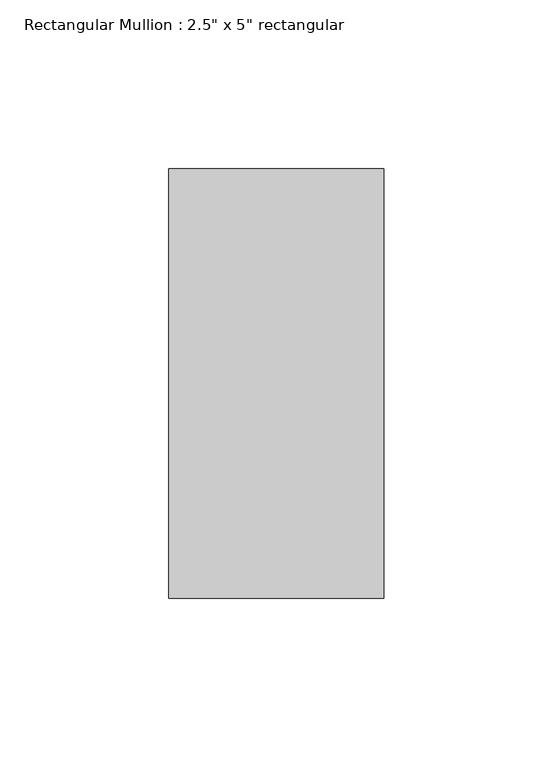
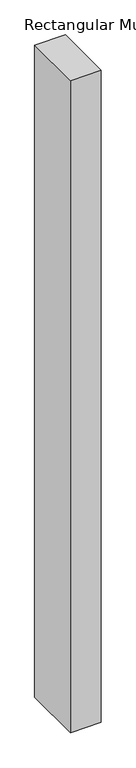
"""IFC4 building model written with IfcOpenShell, lengths in millimetres: member geometry."""

from ifc_helpers import new_model, si_unit, frame, origin, place, context, project, spatial, polyline, outline, extrude, source, transform, mapped, element, save


def member_606b50d7(model_context):
    return source(origin(), model_context, "Body", "SweptSolid", [
        extrude(outline(polyline([(31.75, 63.5), (31.75, -63.5), (-31.75, -63.5), (-31.75, 63.5), (31.75, 63.5)])), frame((0.0, 0.0, -1419.6724956), z_axis=(0.0, 0.0, 1.0), x_axis=(1.0, 0.0, 0.0)), (0.0, 0.0, 1.0), 1419.6724956),
    ])


if __name__ == "__main__":
    model = new_model("IFC4")
    model_context = context("Model", 3, world=origin())
    ifc_project = project(units=[si_unit("LENGTHUNIT", "METRE", prefix="MILLI")], contexts=[model_context])
    site = spatial("IfcSite", under=ifc_project)
    building = spatial("IfcBuilding", under=site)
    placement = place(None, origin())
    member_shape = member_606b50d7(model_context)
    element("IfcMember", 1, ObjectType="Rectangular Mullion : 2.5\" x 5\" rectangular", at=placement, inside=building, context=model_context, shape_type="MappedRepresentation", body=[
        mapped(member_shape, transform((0.0, 0.0, 0.0), x_axis=(1.0, 0.0, 0.0), y_axis=(0.0, 1.0, 0.0), z_axis=(0.0, 0.0, 1.0))),
    ])
    save(model, "model.ifc")

# Revit data of these elements
# Type "Rectangular Mullion : 2.5\" x 5\" rectangular"
#   built-in parameter 1007304 = 0.416667 (stored number, unit not read)
#   built-in parameter 1007301 = 0.104167 (stored number, unit not read)
#   built-in parameter 1007300 = 0.104167 (stored number, unit not read)
# Element 1 (IfcMember, "Rectangular Mullion : 2.5\" x 5\" rectangular")
#   Materials on its faces: "BLACK COLOUR"
# Materials
#   "BLACK COLOUR": class "Generic", colour RGB 120 120 120, transparency 0, Cost = 0
